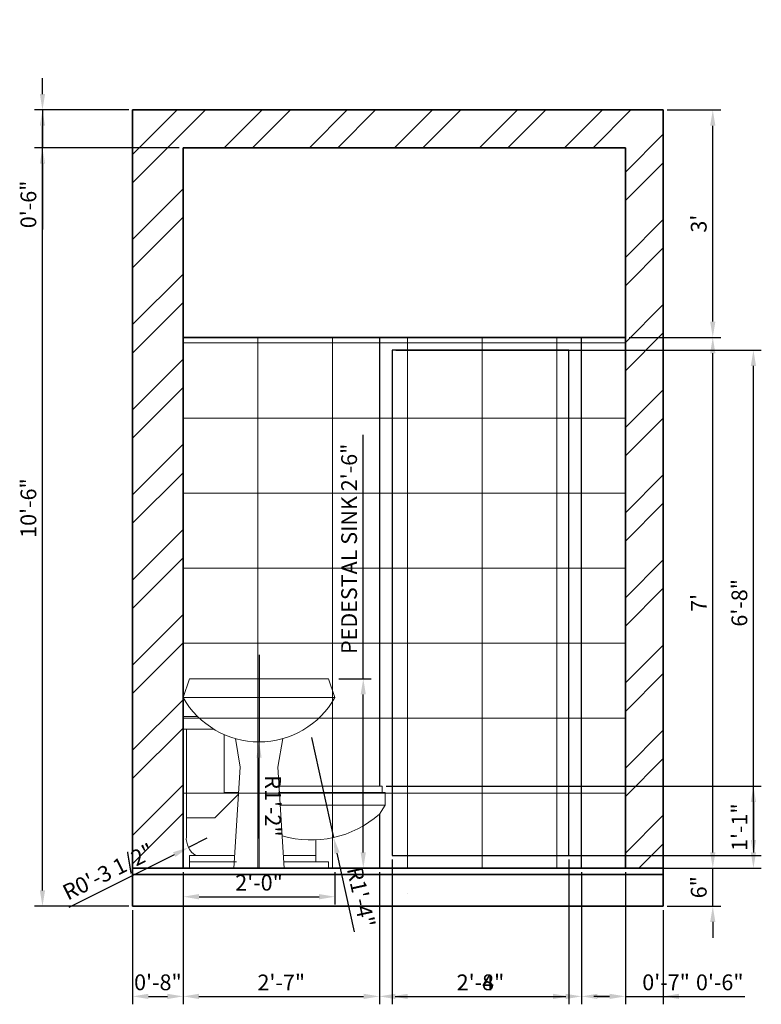
# Model space of a CAD drawing. Units: inches. Extents: x 3082 to 3209, y 1055 to 1366.
# Tile 1 of 2: x 3084 to 3201, y 1055 to 1210. Entities that reach past the tile are written whole.
import ezdxf

# ---------------------------------------------------------------- set-up
doc = ezdxf.new("R2010")
doc.units = ezdxf.units.IN
for name, color, linetype, lineweight in [('A-ANNO-DIMS', 2, 'Continuous', 18), ('A-DOOR', 3, 'Continuous', 25), ('A-ELEV', 7, 'Continuous', 35), ('A-FLOR-FIXT', 9, 'Continuous', 18), ('A-FLOR-PATT', 252, 'Continuous', 13), ('A-WALL-PATT', 8, 'Continuous', 13)]:
    doc.layers.add(name, color=color, linetype=linetype, lineweight=lineweight)
doc.styles.get("Standard").update_dxf_attribs({"font": 'arial.ttf'})
doc.dimstyles.new('ISO-25', dxfattribs={"dimtxt": 2.5, "dimasz": 2.5, "dimexe": 1.25, "dimexo": 0.625, "dimtad": 1, "dimdec": 0, "dimlunit": 3, "dimtxsty": 'Standard', "dimcen": 2.5, "dimadec": 0, "dimazin": 0, "dimtfac": 1, "dimtdec": 0, "dimtmove": 0, "dimatfit": 3, "dimfxl": 1, "dimarcsym": 0})

# ---------------------------------------------------------------- blocks, each defined once
blk = doc.blocks.new('Sink - Pedestal elevation')
for p, q in [((-11, 30), (-12, 27)), ((-11, 30), (11, 30)), ((11, 30), (12, 27)), ((-12, 27), (12, 27)), ((-3, 16), (-3.7523, 20.5139)), ((3.7527, 20.5157), (3, 16)), ((0, 20), (0, 0)), ((-4, 0), (-3, 16)), ((3, 16), (4, 0)), ((-4, 0), (4, 0))]:
    blk.add_line(p, q)
blk.add_arc((0, 33.7857), 13.7857, 209.4871, 330.5129)
blk = doc.blocks.new('*D14')
at = {"layer": 'A-ANNO-DIMS', "color": 0, "lineweight": -2, "transparency": 16777216}
for p, q in [((3193.64, 1078.54), (3193.64, 1081.04)), ((3186.42, 1076.04), (3194.89, 1076.04)), ((3193.64, 1070.04), (3193.64, 1076.04)), ((3186.42, 1070.04), (3194.89, 1070.04)), ((3193.64, 1067.54), (3193.64, 1065.04))]:
    blk.add_line(p, q, dxfattribs=at)
at = {"layer": 'A-ANNO-DIMS', "color": 0, "transparency": 16777216}
for points in [[(3193.22, 1078.54), (3194.05, 1078.54), (3193.64, 1076.04)], [(3193.22, 1067.54), (3194.05, 1067.54), (3193.64, 1070.04)]]:
    blk.add_solid(points, dxfattribs=at)
at = {"layer": 'Defpoints', "color": 0, "transparency": 16777216}
for p in [(3185.8, 1076.04), (3193.64, 1076.04), (3185.8, 1070.04)]:
    blk.add_point(p, dxfattribs=at)
at = {"layer": 'A-ANNO-DIMS', "color": 0, "transparency": 16777216, "insert": (3191.74, 1073.04), "char_height": 2.5, "attachment_point": 5, "rotation": 90}
blk.add_mtext('6"', dxfattribs=at)
blk = doc.blocks.new('*D15')
at = {"layer": 'A-ANNO-DIMS', "color": 0, "lineweight": -2, "transparency": 16777216}
for p, q in [((3180.42, 1160.04), (3194.89, 1160.04)), ((3193.64, 1078.54), (3193.64, 1157.54)), ((3186.42, 1076.04), (3194.89, 1076.04))]:
    blk.add_line(p, q, dxfattribs=at)
at = {"layer": 'A-ANNO-DIMS', "color": 0, "transparency": 16777216}
for points in [[(3193.22, 1157.54), (3194.05, 1157.54), (3193.64, 1160.04)], [(3193.22, 1078.54), (3194.05, 1078.54), (3193.64, 1076.04)]]:
    blk.add_solid(points, dxfattribs=at)
at = {"layer": 'Defpoints', "color": 0, "transparency": 16777216}
for p in [(3179.8, 1160.04), (3193.64, 1160.04), (3185.8, 1076.04)]:
    blk.add_point(p, dxfattribs=at)
at = {"layer": 'A-ANNO-DIMS', "color": 0, "transparency": 16777216, "insert": (3191.76, 1118.04), "char_height": 2.5, "attachment_point": 5, "rotation": 90}
blk.add_mtext("7'", dxfattribs=at)
blk = doc.blocks.new('*D16')
at = {"layer": 'A-ANNO-DIMS', "color": 0, "lineweight": -2, "transparency": 16777216}
for p, q in [((3186.42, 1196.04), (3194.89, 1196.04)), ((3193.64, 1162.54), (3193.64, 1193.54)), ((3194.26, 1160.04), (3194.89, 1160.04))]:
    blk.add_line(p, q, dxfattribs=at)
at = {"layer": 'A-ANNO-DIMS', "color": 0, "transparency": 16777216}
for points in [[(3193.22, 1193.54), (3194.05, 1193.54), (3193.64, 1196.04)], [(3193.22, 1162.54), (3194.05, 1162.54), (3193.64, 1160.04)]]:
    blk.add_solid(points, dxfattribs=at)
at = {"layer": 'Defpoints', "color": 0, "transparency": 16777216}
for p in [(3185.8, 1196.04), (3193.64, 1196.04), (3193.64, 1160.04)]:
    blk.add_point(p, dxfattribs=at)
at = {"layer": 'A-ANNO-DIMS', "color": 0, "transparency": 16777216, "insert": (3191.74, 1178.04), "char_height": 2.5, "attachment_point": 5, "rotation": 90}
blk.add_mtext("3'", dxfattribs=at)
blk = doc.blocks.new('*D22')
at = {"layer": 'A-ANNO-DIMS', "color": 0, "lineweight": -2, "transparency": 16777216}
for p, q in [((3138.31, 1106.04), (3138.31, 1144.65)), ((3134.43, 1106.04), (3139.56, 1106.04)), ((3138.31, 1078.54), (3138.31, 1103.54)), ((3134.43, 1076.04), (3139.56, 1076.04))]:
    blk.add_line(p, q, dxfattribs=at)
at = {"layer": 'A-ANNO-DIMS', "color": 0, "transparency": 16777216}
for points in [[(3137.89, 1103.54), (3138.72, 1103.54), (3138.31, 1106.04)], [(3137.89, 1078.54), (3138.72, 1078.54), (3138.31, 1076.04)]]:
    blk.add_solid(points, dxfattribs=at)
at = {"layer": 'Defpoints', "color": 0, "transparency": 16777216}
for p in [(3133.81, 1106.04), (3138.31, 1106.04), (3133.81, 1076.04)]:
    blk.add_point(p, dxfattribs=at)
at = {"layer": 'A-ANNO-DIMS', "color": 0, "transparency": 16777216, "insert": (3136.39, 1126.59), "char_height": 2.5, "attachment_point": 5, "rotation": 90}
blk.add_mtext('PEDESTAL SINK 2\'-6"', dxfattribs=at)
blk = doc.blocks.new('*D23')
at = {"layer": 'A-ANNO-DIMS', "color": 0, "lineweight": -2, "transparency": 16777216}
for p, q in [((3109.81, 1075.42), (3109.81, 1070.29)), ((3133.81, 1075.42), (3133.81, 1070.29)), ((3112.31, 1071.54), (3131.31, 1071.54))]:
    blk.add_line(p, q, dxfattribs=at)
at = {"layer": 'A-ANNO-DIMS', "color": 0, "transparency": 16777216}
for points in [[(3112.31, 1071.96), (3112.31, 1071.12), (3109.81, 1071.54)], [(3131.31, 1071.96), (3131.31, 1071.12), (3133.81, 1071.54)]]:
    blk.add_solid(points, dxfattribs=at)
at = {"layer": 'Defpoints', "color": 0, "transparency": 16777216}
for p in [(3109.81, 1076.04), (3133.81, 1076.04), (3133.81, 1071.54)]:
    blk.add_point(p, dxfattribs=at)
at = {"layer": 'A-ANNO-DIMS', "color": 0, "transparency": 16777216, "insert": (3121.81, 1073.44), "char_height": 2.5, "attachment_point": 5}
blk.add_mtext('2\'-0"', dxfattribs=at)
blk = doc.blocks.new('*D31')
at = {"layer": 'A-ANNO-DIMS', "color": 0, "lineweight": -2, "transparency": 16777216}
for p, q in [((3109.8, 1075.42), (3109.8, 1054.52)), ((3101.8, 1069.42), (3101.8, 1054.52)), ((3104.3, 1055.77), (3107.3, 1055.77))]:
    blk.add_line(p, q, dxfattribs=at)
at = {"layer": 'A-ANNO-DIMS', "color": 0, "transparency": 16777216}
for points in [[(3104.3, 1056.18), (3104.3, 1055.35), (3101.8, 1055.77)], [(3107.3, 1056.18), (3107.3, 1055.35), (3109.8, 1055.77)]]:
    blk.add_solid(points, dxfattribs=at)
at = {"layer": 'Defpoints', "color": 0, "transparency": 16777216}
for p in [(3109.8, 1076.04), (3101.8, 1070.04), (3109.8, 1055.77)]:
    blk.add_point(p, dxfattribs=at)
at = {"layer": 'A-ANNO-DIMS', "color": 0, "transparency": 16777216, "insert": (3105.8, 1057.67), "char_height": 2.5, "attachment_point": 5}
blk.add_mtext('0\'-8"', dxfattribs=at)
blk = doc.blocks.new('*D32')
at = {"layer": 'A-ANNO-DIMS', "color": 0, "lineweight": -2, "transparency": 16777216}
for p, q in [((3109.8, 1075.42), (3109.8, 1054.52)), ((3140.86, 1075.42), (3140.86, 1054.52)), ((3112.3, 1055.77), (3138.36, 1055.77))]:
    blk.add_line(p, q, dxfattribs=at)
at = {"layer": 'A-ANNO-DIMS', "color": 0, "transparency": 16777216}
for points in [[(3112.3, 1056.18), (3112.3, 1055.35), (3109.8, 1055.77)], [(3138.36, 1056.18), (3138.36, 1055.35), (3140.86, 1055.77)]]:
    blk.add_solid(points, dxfattribs=at)
at = {"layer": 'Defpoints', "color": 0, "transparency": 16777216}
for p in [(3109.8, 1076.04), (3140.86, 1076.04), (3140.86, 1055.77)]:
    blk.add_point(p, dxfattribs=at)
at = {"layer": 'A-ANNO-DIMS', "color": 0, "transparency": 16777216, "insert": (3125.33, 1057.65), "char_height": 2.5, "attachment_point": 5}
blk.add_mtext('2\'-7"', dxfattribs=at)
blk = doc.blocks.new('*D33')
at = {"layer": 'A-ANNO-DIMS', "color": 0, "lineweight": -2, "transparency": 16777216}
for p, q in [((3140.86, 1075.42), (3140.86, 1054.52)), ((3172.86, 1075.42), (3172.86, 1054.52)), ((3143.36, 1055.77), (3170.36, 1055.77))]:
    blk.add_line(p, q, dxfattribs=at)
at = {"layer": 'A-ANNO-DIMS', "color": 0, "transparency": 16777216}
for points in [[(3143.36, 1056.18), (3143.36, 1055.35), (3140.86, 1055.77)], [(3170.36, 1056.18), (3170.36, 1055.35), (3172.86, 1055.77)]]:
    blk.add_solid(points, dxfattribs=at)
at = {"layer": 'Defpoints', "color": 0, "transparency": 16777216}
for p in [(3140.86, 1076.04), (3172.86, 1076.04), (3172.86, 1055.77)]:
    blk.add_point(p, dxfattribs=at)
at = {"layer": 'A-ANNO-DIMS', "color": 0, "transparency": 16777216, "insert": (3156.86, 1057.67), "char_height": 2.5, "attachment_point": 5}
blk.add_mtext('2\'-8"', dxfattribs=at)
blk = doc.blocks.new('*D34')
at = {"layer": 'A-ANNO-DIMS', "color": 0, "lineweight": -2, "transparency": 16777216}
for p, q in [((3172.86, 1075.42), (3172.86, 1054.52)), ((3179.8, 1075.42), (3179.8, 1054.52)), ((3175.36, 1055.77), (3177.3, 1055.77)), ((3179.8, 1055.77), (3190.19, 1055.77))]:
    blk.add_line(p, q, dxfattribs=at)
at = {"layer": 'A-ANNO-DIMS', "color": 0, "transparency": 16777216}
for points in [[(3175.36, 1056.18), (3175.36, 1055.35), (3172.86, 1055.77)], [(3177.3, 1056.18), (3177.3, 1055.35), (3179.8, 1055.77)]]:
    blk.add_solid(points, dxfattribs=at)
at = {"layer": 'Defpoints', "color": 0, "transparency": 16777216}
for p in [(3172.86, 1076.04), (3179.8, 1076.04), (3179.8, 1055.77)]:
    blk.add_point(p, dxfattribs=at)
at = {"layer": 'A-ANNO-DIMS', "color": 0, "transparency": 16777216, "insert": (3186.24, 1057.67), "char_height": 2.5, "attachment_point": 5}
blk.add_mtext('0\'-7"', dxfattribs=at)
blk = doc.blocks.new('*D35')
at = {"layer": 'A-ANNO-DIMS', "color": 0, "lineweight": -2, "transparency": 16777216}
for p, q in [((3179.8, 1075.42), (3179.8, 1054.52)), ((3185.8, 1069.42), (3185.8, 1054.52)), ((3177.3, 1055.77), (3174.8, 1055.77)), ((3179.8, 1055.77), (3185.8, 1055.77)), ((3188.3, 1055.77), (3198.69, 1055.77))]:
    blk.add_line(p, q, dxfattribs=at)
at = {"layer": 'A-ANNO-DIMS', "color": 0, "transparency": 16777216}
for points in [[(3177.3, 1056.18), (3177.3, 1055.35), (3179.8, 1055.77)], [(3188.3, 1056.18), (3188.3, 1055.35), (3185.8, 1055.77)]]:
    blk.add_solid(points, dxfattribs=at)
at = {"layer": 'Defpoints', "color": 0, "transparency": 16777216}
for p in [(3179.8, 1076.04), (3185.8, 1070.04), (3185.8, 1055.77)]:
    blk.add_point(p, dxfattribs=at)
at = {"layer": 'A-ANNO-DIMS', "color": 0, "transparency": 16777216, "insert": (3194.74, 1057.67), "char_height": 2.5, "attachment_point": 5}
blk.add_mtext('0\'-6"', dxfattribs=at)
blk = doc.blocks.new('*D36')
at = {"layer": 'A-ANNO-DIMS', "color": 0, "lineweight": -2, "transparency": 16777216}
for p, q in [((3101.17, 1196.04), (3086.27, 1196.04)), ((3087.52, 1072.54), (3087.52, 1193.54)), ((3101.17, 1070.04), (3086.27, 1070.04))]:
    blk.add_line(p, q, dxfattribs=at)
at = {"layer": 'A-ANNO-DIMS', "color": 0, "transparency": 16777216}
for points in [[(3087.11, 1193.54), (3087.94, 1193.54), (3087.52, 1196.04)], [(3087.11, 1072.54), (3087.94, 1072.54), (3087.52, 1070.04)]]:
    blk.add_solid(points, dxfattribs=at)
at = {"layer": 'Defpoints', "color": 0, "transparency": 16777216}
for p in [(3087.52, 1196.04), (3101.8, 1196.04), (3101.8, 1070.04)]:
    blk.add_point(p, dxfattribs=at)
at = {"layer": 'A-ANNO-DIMS', "color": 0, "transparency": 16777216, "insert": (3085.62, 1133.04), "char_height": 2.5, "attachment_point": 5, "rotation": 90}
blk.add_mtext('10\'-6"', dxfattribs=at)
blk = doc.blocks.new('*D37')
at = {"layer": 'A-ANNO-DIMS', "color": 0, "lineweight": -2, "transparency": 16777216}
for p, q in [((3087.52, 1198.54), (3087.52, 1201.04)), ((3101.17, 1196.04), (3086.27, 1196.04)), ((3087.52, 1196.04), (3087.52, 1190.04)), ((3109.17, 1190.04), (3086.27, 1190.04)), ((3087.52, 1187.54), (3087.52, 1177.14))]:
    blk.add_line(p, q, dxfattribs=at)
at = {"layer": 'A-ANNO-DIMS', "color": 0, "transparency": 16777216}
for points in [[(3087.11, 1198.54), (3087.94, 1198.54), (3087.52, 1196.04)], [(3087.11, 1187.54), (3087.94, 1187.54), (3087.52, 1190.04)]]:
    blk.add_solid(points, dxfattribs=at)
at = {"layer": 'Defpoints', "color": 0, "transparency": 16777216}
for p in [(3101.8, 1196.04), (3087.52, 1190.04), (3109.8, 1190.04)]:
    blk.add_point(p, dxfattribs=at)
at = {"layer": 'A-ANNO-DIMS', "color": 0, "transparency": 16777216, "insert": (3085.62, 1181.09), "char_height": 2.5, "attachment_point": 5, "rotation": 90}
blk.add_mtext('0\'-6"', dxfattribs=at)
blk = doc.blocks.new('*D38')
at = {"layer": 'A-ANNO-DIMS', "color": 0, "lineweight": -2, "transparency": 16777216}
for p, q in [((3143.48, 1158.04), (3201.32, 1158.04)), ((3200.07, 1080.54), (3200.07, 1155.54)), ((3143.48, 1078.04), (3201.32, 1078.04))]:
    blk.add_line(p, q, dxfattribs=at)
at = {"layer": 'A-ANNO-DIMS', "color": 0, "transparency": 16777216}
for points in [[(3199.66, 1155.54), (3200.49, 1155.54), (3200.07, 1158.04)], [(3199.66, 1080.54), (3200.49, 1080.54), (3200.07, 1078.04)]]:
    blk.add_solid(points, dxfattribs=at)
at = {"layer": 'Defpoints', "color": 0, "transparency": 16777216}
for p in [(3142.86, 1158.04), (3200.07, 1158.04), (3142.86, 1078.04)]:
    blk.add_point(p, dxfattribs=at)
at = {"layer": 'A-ANNO-DIMS', "color": 0, "transparency": 16777216, "insert": (3198.17, 1118.04), "char_height": 2.5, "attachment_point": 5, "rotation": 90}
blk.add_mtext('6\'-8"', dxfattribs=at)
blk = doc.blocks.new('*D39')
at = {"layer": 'A-ANNO-DIMS', "color": 0, "lineweight": -2, "transparency": 16777216}
for p, q in [((3142.86, 1077.42), (3142.86, 1054.52)), ((3170.86, 1077.42), (3170.86, 1054.52)), ((3145.36, 1055.77), (3168.36, 1055.77))]:
    blk.add_line(p, q, dxfattribs=at)
at = {"layer": 'A-ANNO-DIMS', "color": 0, "transparency": 16777216}
for points in [[(3145.36, 1056.18), (3145.36, 1055.35), (3142.86, 1055.77)], [(3168.36, 1056.18), (3168.36, 1055.35), (3170.86, 1055.77)]]:
    blk.add_solid(points, dxfattribs=at)
at = {"layer": 'Defpoints', "color": 0, "transparency": 16777216}
for p in [(3142.86, 1078.04), (3170.86, 1078.04), (3170.86, 1055.77)]:
    blk.add_point(p, dxfattribs=at)
at = {"layer": 'A-ANNO-DIMS', "color": 0, "transparency": 16777216, "insert": (3156.86, 1057.65), "char_height": 2.5, "attachment_point": 5}
blk.add_mtext('2\'-4"', dxfattribs=at)
blk = doc.blocks.new('*D40')
at = {"layer": 'A-ANNO-DIMS', "color": 0, "lineweight": -2, "transparency": 16777216}
for p, q in [((3141.92, 1089.04), (3201.32, 1089.04)), ((3200.07, 1086.54), (3200.07, 1078.54)), ((3141.48, 1076.04), (3201.32, 1076.04))]:
    blk.add_line(p, q, dxfattribs=at)
at = {"layer": 'A-ANNO-DIMS', "color": 0, "transparency": 16777216}
for points in [[(3199.66, 1086.54), (3200.49, 1086.54), (3200.07, 1089.04)], [(3199.66, 1078.54), (3200.49, 1078.54), (3200.07, 1076.04)]]:
    blk.add_solid(points, dxfattribs=at)
at = {"layer": 'Defpoints', "color": 0, "transparency": 16777216}
for p in [(3141.3, 1089.04), (3140.86, 1076.04), (3200.07, 1076.04)]:
    blk.add_point(p, dxfattribs=at)
at = {"layer": 'A-ANNO-DIMS', "color": 0, "transparency": 16777216, "insert": (3198.19, 1082.54), "char_height": 2.5, "attachment_point": 5, "rotation": 90}
blk.add_mtext('1\'-1"', dxfattribs=at)
blk = doc.blocks.new('*D44')
at = {"layer": 'A-ANNO-DIMS', "color": 0, "lineweight": -2, "transparency": 16777216}
for p, q in [((3130.09, 1096.74), (3133.62, 1080.9)), ((3136.94, 1065.97), (3134.16, 1078.45))]:
    blk.add_line(p, q, dxfattribs=at)
at = {"layer": 'A-ANNO-DIMS', "color": 0, "transparency": 16777216}
blk.add_solid([(3134.57, 1078.55), (3133.75, 1078.36), (3133.62, 1080.9)], dxfattribs=at)
at = {"layer": 'Defpoints', "color": 0, "transparency": 16777216}
for p in [(3130.09, 1096.74), (3133.62, 1080.9)]:
    blk.add_point(p, dxfattribs=at)
at = {"layer": 'A-ANNO-DIMS', "color": 0, "transparency": 16777216, "insert": (3137.65, 1071.4), "char_height": 2.5, "attachment_point": 5, "rotation": 282.5409}
blk.add_mtext('R1\'-4"', dxfattribs=at)
blk = doc.blocks.new('*D45')
at = {"layer": 'A-ANNO-DIMS', "color": 0, "lineweight": -2, "transparency": 16777216}
for p, q in [((3121.81, 1109.83), (3121.81, 1096.04)), ((3121.81, 1080.75), (3121.81, 1093.54))]:
    blk.add_line(p, q, dxfattribs=at)
at = {"layer": 'A-ANNO-DIMS', "color": 0, "transparency": 16777216}
blk.add_solid([(3122.22, 1093.54), (3121.39, 1093.54), (3121.81, 1096.04)], dxfattribs=at)
at = {"layer": 'Defpoints', "color": 0, "transparency": 16777216}
for p in [(3121.81, 1109.83), (3121.81, 1096.04)]:
    blk.add_point(p, dxfattribs=at)
at = {"layer": 'A-ANNO-DIMS', "color": 0, "transparency": 16777216, "insert": (3123.69, 1085.9), "char_height": 2.5, "attachment_point": 5, "rotation": 270.0008}
blk.add_mtext('R1\'-2"', dxfattribs=at)
blk = doc.blocks.new('*D46')
at = {"layer": 'A-ANNO-DIMS', "color": 0, "lineweight": -2, "transparency": 16777216}
for p, q in [((3113.55, 1080.79), (3110.63, 1079.33)), ((3091.75, 1069.89), (3108.4, 1078.21))]:
    blk.add_line(p, q, dxfattribs=at)
at = {"layer": 'A-ANNO-DIMS', "color": 0, "transparency": 16777216}
blk.add_solid([(3108.21, 1078.59), (3108.58, 1077.84), (3110.63, 1079.33)], dxfattribs=at)
at = {"layer": 'Defpoints', "color": 0, "transparency": 16777216}
for p in [(3113.55, 1080.79), (3110.63, 1079.33)]:
    blk.add_point(p, dxfattribs=at)
at = {"layer": 'A-ANNO-DIMS', "color": 0, "transparency": 16777216, "insert": (3098.1, 1075.21), "char_height": 2.5, "attachment_point": 5, "rotation": 26.5643}
blk.add_mtext('R0\'-3 1/2"', dxfattribs=at)

msp = doc.modelspace()

# ---------------------------------------------------------------- hatches: boundary and pattern name
at = {"layer": 'A-WALL-PATT'}
h = msp.add_hatch(dxfattribs=at)
h.set_pattern_fill('ANSI32', color=256)
h.paths.add_polyline_path([(3185.8, 1196.04), (3101.8, 1196.04), (3101.8, 1076.04), (3109.8, 1076.04), (3109.8, 1160.04), (3109.8, 1190.04), (3179.8, 1190.04), (3179.8, 1076.04), (3185.8, 1076.04)])
h.paths.add_polyline_path([(3185.8, 1348.24), (3155.8, 1348.24), (3155.8, 1342.24), (3179.8, 1342.24), (3179.8, 1246.24), (3173.53, 1246.24), (3173.53, 1240.24), (3185.8, 1240.24)])
h.paths.add_polyline_path([(3107.8, 1342.24), (3131.8, 1342.24), (3131.8, 1348.24), (3101.8, 1348.24), (3101.8, 1240.24), (3141.53, 1240.24), (3141.53, 1246.24), (3107.8, 1246.24)])
h = msp.add_hatch(dxfattribs=at)
h.set_pattern_fill('AR-CONC', color=256, scale=0.4)
h.paths.add_polyline_path([(3185.8, 1075.04), (3101.8, 1075.04), (3101.8, 1070.04), (3185.8, 1070.04)])

# ---------------------------------------------------------------- linework, layer by layer
at = {"layer": 'A-DOOR'}
msp.add_line((3170.86, 1158.04), (3142.86, 1158.04), dxfattribs=at)
for points in [[(3140.86, 1084.59), (3140.86, 1076.04), (3172.86, 1076.04), (3172.86, 1160.04), (3140.86, 1160.04), (3140.86, 1089.04)], [(3142.86, 1085.56), (3142.86, 1078.04), (3170.86, 1078.04), (3170.86, 1158.04), (3142.86, 1158.04), (3142.86, 1078.04)]]:
    msp.add_lwpolyline(points, dxfattribs=at)
at = {"layer": 'A-ELEV'}
for p, q in [((3101.8, 1070.04), (3101.8, 1196.04)), ((3185.8, 1196.04), (3101.8, 1196.04)), ((3185.8, 1070.04), (3185.8, 1196.04)), ((3109.8, 1160.04), (3109.8, 1190.04)), ((3179.8, 1190.04), (3109.8, 1190.04)), ((3179.8, 1076.04), (3179.8, 1190.04)), ((3179.8, 1160.04), (3109.8, 1160.04)), ((3185.8, 1076.04), (3101.8, 1076.04)), ((3185.8, 1075.04), (3101.8, 1075.04)), ((3185.8, 1070.04), (3101.8, 1070.04))]:
    msp.add_line(p, q, dxfattribs=at)
at = {"layer": 'A-ELEV', "transparency": 33554513}
msp.add_lwpolyline([(3109.8, 1076.04), (3179.8, 1076.04), (3179.8, 1160.04), (3109.8, 1160.04)], close=True, dxfattribs=at)
at = {"layer": 'A-FLOR-FIXT'}
for p, q in [((3110.3, 1081.04), (3110.3, 1098.04)), ((3141.8, 1086.04), (3140.86, 1084.59)), ((3109.8, 1076.04), (3109.8, 1084.04)), ((3130.8, 1080.54), (3130.8, 1078.04)), ((3130.8, 1078.04), (3125.68, 1078.04))]:
    msp.add_line(p, q, dxfattribs=at)
for points in [[(3109.8, 1084.04), (3109.8, 1160.04)], [(3114.66, 1098.04), (3109.8, 1098.04), (3109.8, 1100.04), (3112.1, 1100.04)], [(3116.3, 1097.19), (3116.3, 1088.04), (3118.56, 1088.04)], [(3118.54, 1087.79), (3114.8, 1084.04), (3110.3, 1084.04)], [(3141.3, 1088.04), (3141.3, 1089.04), (3125, 1089.04)], [(3125.06, 1088.04), (3141.8, 1088.04), (3141.8, 1086.04), (3125.18, 1086.04)], [(3130.8, 1077.04), (3130.8, 1078.04), (3130.8, 1080.58)], [(3117.93, 1078.04), (3110.8, 1078.04), (3110.8, 1077.04)], [(3118.16, 1076.04), (3110.8, 1076.04), (3110.8, 1077.04), (3118.23, 1077.04)], [(3125.75, 1077.04), (3132.8, 1077.04), (3132.8, 1076.04), (3124.8, 1076.04)]]:
    msp.add_lwpolyline(points, dxfattribs=at)
for centre, radius, start, end in [((3130.09, 1096.74), 16.23, 253.514, 311.5682), ((3113.55, 1080.79), 3.26, 175.6013, 237.5288)]:
    msp.add_arc(centre, radius, start, end, dxfattribs=at)
at = {"layer": 'A-FLOR-PATT', "transparency": 33554513}
for p, q in [((3109.8, 1160.04), (3109.8, 1076.04)), ((3179.8, 1159.17), (3109.8, 1159.17)), ((3121.63, 1160.04), (3121.63, 1076.04)), ((3133.46, 1160.04), (3133.46, 1076.04)), ((3145.3, 1160.04), (3145.3, 1076.04)), ((3157.13, 1160.04), (3157.13, 1076.04)), ((3168.96, 1160.04), (3168.96, 1076.04)), ((3179.8, 1147.29), (3109.8, 1147.29)), ((3179.8, 1135.42), (3109.8, 1135.42)), ((3179.8, 1123.54), (3109.8, 1123.54)), ((3179.8, 1111.67), (3109.8, 1111.67)), ((3179.8, 1099.79), (3109.8, 1099.79)), ((3179.8, 1087.92), (3109.8, 1087.92))]:
    msp.add_line(p, q, dxfattribs=at)
msp.add_lwpolyline([(3109.8, 1076.04), (3179.8, 1076.04)], dxfattribs=at)

# ---------------------------------------------------------------- block references
at = {"layer": 'A-FLOR-FIXT'}
msp.add_blockref('Sink - Pedestal elevation', (3121.81, 1076.04), dxfattribs=at)

# ---------------------------------------------------------------- dimensions: what is measured, and where the dimension line sits
at = {"layer": 'A-ANNO-DIMS'}
for base, p1, p2, override, picture, middle in [((3087.52, 1190.04), (3101.8, 1196.04), (3109.8, 1190.04), {"dimdec": 1, "dimlfac": 1, "dimrnd": 0, "dimzin": 1, "dimdsep": 46, "dimlunit": 4, "dimfrac": 2}, '*D37', (3085.62, 1181.09)), ((3087.52, 1196.04), (3101.8, 1070.04), (3101.8, 1196.04), {"dimdec": 1, "dimlfac": 1, "dimrnd": 0, "dimzin": 1, "dimdsep": 46, "dimlunit": 4, "dimfrac": 2}, '*D36', (3085.62, 1133.04)), ((3193.64, 1196.04), (3193.64, 1160.04), (3185.8, 1196.04), {"dimclrd": 0, "dimclre": 0, "dimclrt": 0}, '*D16', (3191.74, 1178.04)), ((3193.64, 1160.04), (3185.8, 1076.04), (3179.8, 1160.04), {"dimclrd": 0, "dimclre": 0, "dimclrt": 0}, '*D15', (3191.76, 1118.04)), ((3200.07, 1158.04), (3142.86, 1078.04), (3142.86, 1158.04), {"dimdec": 1, "dimlfac": 1, "dimrnd": 0, "dimzin": 1, "dimdsep": 46, "dimlunit": 4, "dimfrac": 2}, '*D38', (3198.17, 1118.04)), ((3200.07, 1076.04), (3141.3, 1089.04), (3140.86, 1076.04), {"dimdec": 1, "dimlfac": 1, "dimrnd": 0, "dimzin": 1, "dimdsep": 46, "dimlunit": 4, "dimfrac": 2}, '*D40', (3198.19, 1082.54)), ((3193.64, 1076.04), (3185.8, 1070.04), (3185.8, 1076.04), {"dimclrd": 0, "dimclre": 0, "dimclrt": 0}, '*D14', (3191.74, 1073.04))]:
    dim = msp.add_linear_dim(base=base, p1=p1, p2=p2, angle=90, dimstyle='ISO-25', override=override, dxfattribs=at)
    dim.commit()
    dim.dimension.update_dxf_attribs({"geometry": picture, "text_midpoint": middle})
dim = msp.add_linear_dim(base=(3138.31, 1106.04), p1=(3133.81, 1076.04), p2=(3133.81, 1106.04), angle=90, text='PEDESTAL SINK <>', dimstyle='ISO-25', override={"dimdec": 1, "dimrnd": 0, "dimzin": 1, "dimlunit": 4, "dimfrac": 2}, dxfattribs=at)
dim.commit()
dim.dimension.update_dxf_attribs({"geometry": '*D22', "text_midpoint": (3136.39, 1126.59)})
for center, mpoint, picture, middle in [((3121.81, 1109.83), (3121.81, 1096.04), '*D45', (3123.69, 1085.9)), ((3130.09, 1096.74), (3133.62, 1080.9), '*D44', (3137.65, 1071.4)), ((3113.55, 1080.79), (3110.63, 1079.33), '*D46', (3098.1, 1075.21))]:
    dim = msp.add_radius_dim(center=center, mpoint=mpoint, dimstyle='ISO-25', override={"dimdec": 1, "dimlfac": 1, "dimrnd": 0, "dimzin": 1, "dimdsep": 46, "dimlunit": 4, "dimfrac": 2}, dxfattribs=at)
    dim.commit()
    dim.dimension.update_dxf_attribs({"geometry": picture, "text_midpoint": middle})
for base, p1, p2, override, picture, middle in [((3170.86, 1055.77), (3142.86, 1078.04), (3170.86, 1078.04), {"dimdec": 1, "dimlfac": 1, "dimrnd": 0, "dimzin": 1, "dimdsep": 46, "dimlunit": 4, "dimfrac": 2}, '*D39', (3156.86, 1057.65)), ((3109.8, 1055.77), (3101.8, 1070.04), (3109.8, 1076.04), {"dimdec": 1, "dimlfac": 1, "dimrnd": 0, "dimzin": 1, "dimdsep": 46, "dimlunit": 4, "dimfrac": 2}, '*D31', (3105.8, 1057.67)), ((3140.86, 1055.77), (3109.8, 1076.04), (3140.86, 1076.04), {"dimdec": 1, "dimlfac": 1, "dimrnd": 0, "dimzin": 1, "dimdsep": 46, "dimlunit": 4, "dimfrac": 2}, '*D32', (3125.33, 1057.65)), ((3133.81, 1071.54), (3109.81, 1076.04), (3133.81, 1076.04), {"dimdec": 1, "dimrnd": 0, "dimzin": 1, "dimlunit": 4, "dimfrac": 2}, '*D23', (3121.81, 1073.44)), ((3172.86, 1055.77), (3140.86, 1076.04), (3172.86, 1076.04), {"dimdec": 1, "dimlfac": 1, "dimrnd": 0, "dimzin": 1, "dimdsep": 46, "dimlunit": 4, "dimfrac": 2}, '*D33', (3156.86, 1057.67)), ((3179.8, 1055.77), (3172.86, 1076.04), (3179.8, 1076.04), {"dimdec": 1, "dimlfac": 1, "dimrnd": 0, "dimzin": 1, "dimdsep": 46, "dimlunit": 4, "dimfrac": 2}, '*D34', (3186.24, 1057.67)), ((3185.8, 1055.77), (3179.8, 1076.04), (3185.8, 1070.04), {"dimdec": 1, "dimlfac": 1, "dimrnd": 0, "dimzin": 1, "dimdsep": 46, "dimlunit": 4, "dimfrac": 2}, '*D35', (3194.74, 1057.67))]:
    dim = msp.add_linear_dim(base=base, p1=p1, p2=p2, dimstyle='ISO-25', override=override, dxfattribs=at)
    dim.commit()
    dim.dimension.update_dxf_attribs({"geometry": picture, "text_midpoint": middle})

doc.saveas('drawing.dxf')
